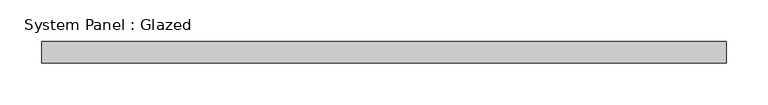
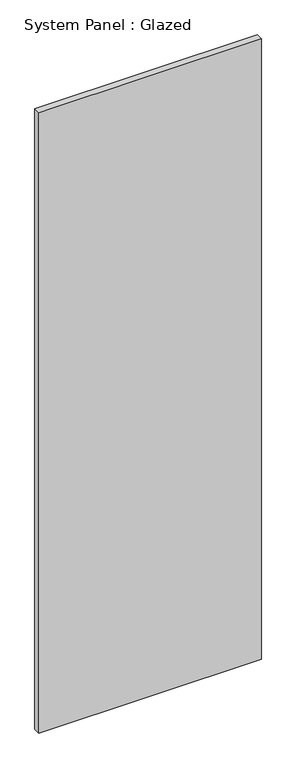
"""IFC4 building model written with IfcOpenShell, lengths in millimetres: plate geometry, System Panel : Glazed."""

from ifc_helpers import new_model, si_unit, origin, origin_with_axes, place, context, project, spatial, polyline, outline, extrude, source, transform, mapped, element, save


def system_panel_glazed_bafc467c(model_context):
    return source(origin(), model_context, "Body", "SweptSolid", [
        extrude(outline(polyline([(409.575, 19.05), (-409.575, 19.05), (-409.575, 44.45), (409.575, 44.45), (409.575, 19.05)])), origin_with_axes(), (0.0, 0.0, 1.0), 2413.0),
    ])


if __name__ == "__main__":
    model = new_model("IFC4")
    model_context = context("Model", 3, world=origin())
    ifc_project = project(units=[si_unit("LENGTHUNIT", "METRE", prefix="MILLI")], contexts=[model_context])
    site = spatial("IfcSite", under=ifc_project)
    building = spatial("IfcBuilding", under=site)
    placement = place(None, origin())
    system_panel_glazed_shape = system_panel_glazed_bafc467c(model_context)
    element("IfcPlate", 1, ObjectType="System Panel : Glazed", at=placement, inside=building, context=model_context, shape_type="MappedRepresentation", body=[
        mapped(system_panel_glazed_shape, transform((0.0, 0.0, 0.0), x_axis=(1.0, 0.0, 0.0), y_axis=(0.0, 1.0, 0.0), z_axis=(0.0, 0.0, 1.0))),
    ])
    save(model, "model.ifc")

# Revit data of these elements
# Type "System Panel : Glazed"
#   Construction Type Id = "GSP4R"
#   Analytic Construction = "1/8 in Pilkington single glazing"
#   Visual Light Transmittance = 0.9
#   Solar Heat Gain Coefficient = 0.86
#   Heat Transfer Coefficient (U) = 1.18115 BTU/(h·ft²·°F)
# Element 1 (IfcPlate, "System Panel : Glazed")
#   Materials on its faces: "Glass"
# Materials
#   "Glass": class "Glass", colour RGB 0 128 192, transparency 0.75, Description = "Soda Lime Glass", Cost = 0
